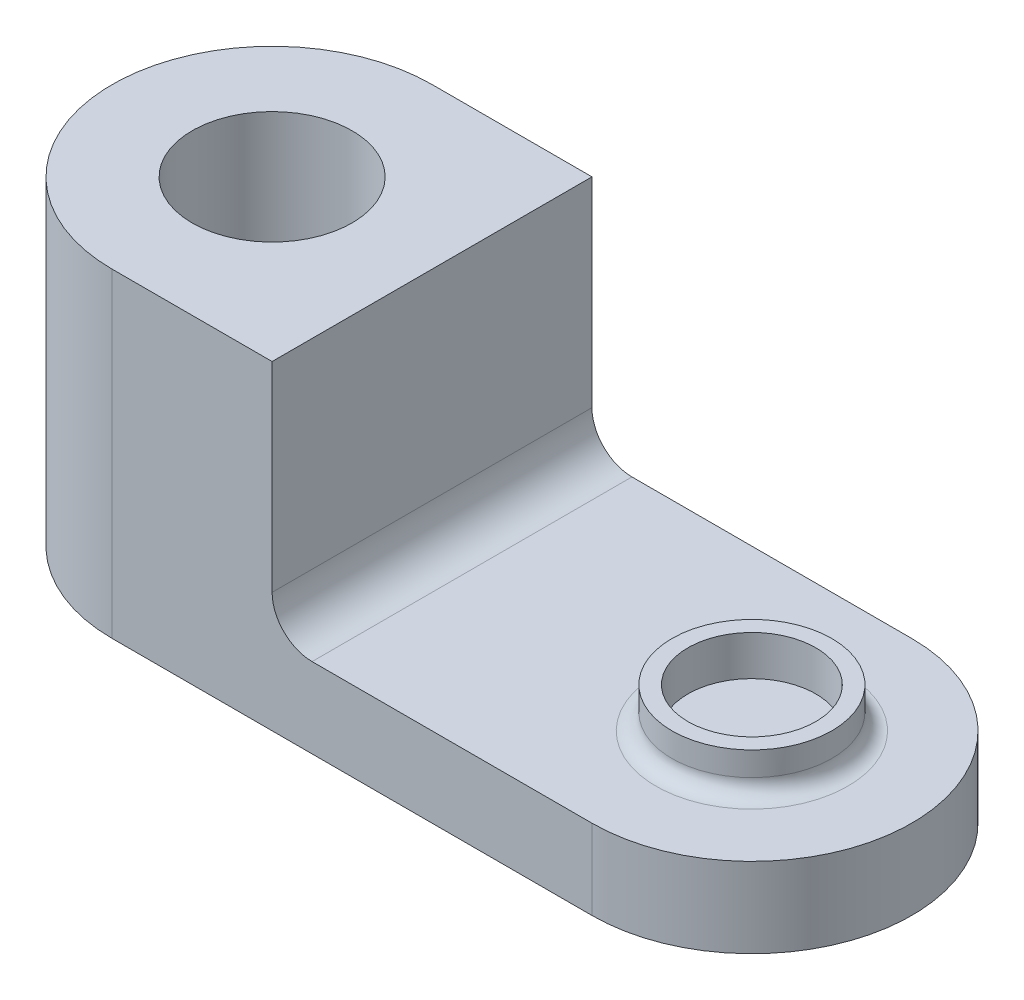
ISO-10303-21;
HEADER;
FILE_DESCRIPTION(('STEP AP214'),'2;1');
FILE_NAME('part.step','',(''),(''),'','','');
FILE_SCHEMA(('AUTOMOTIVE_DESIGN { 1 0 10303 214 1 1 1 1 }'));
ENDSEC;
DATA;
#1=APPLICATION_CONTEXT('core data for automotive mechanical design processes');
#2=APPLICATION_PROTOCOL_DEFINITION('international standard','automotive_design',2000,#1);
#3=PRODUCT_CONTEXT('',#1,'mechanical');
#4=PRODUCT('Part','Part','',(#3));
#5=PRODUCT_RELATED_PRODUCT_CATEGORY('part','',(#4));
#6=PRODUCT_DEFINITION_FORMATION('','',#4);
#7=PRODUCT_DEFINITION_CONTEXT('part definition',#1,'design');
#8=PRODUCT_DEFINITION('design','',#6,#7);
#9=PRODUCT_DEFINITION_SHAPE('','',#8);
#10=(LENGTH_UNIT() NAMED_UNIT(*) SI_UNIT(.MILLI.,.METRE.));
#11=(NAMED_UNIT(*) PLANE_ANGLE_UNIT() SI_UNIT($,.RADIAN.));
#12=(NAMED_UNIT(*) SI_UNIT($,.STERADIAN.) SOLID_ANGLE_UNIT());
#13=UNCERTAINTY_MEASURE_WITH_UNIT(LENGTH_MEASURE(1.E-05),#10,'distance_accuracy_value','');
#14=(GEOMETRIC_REPRESENTATION_CONTEXT(3) GLOBAL_UNCERTAINTY_ASSIGNED_CONTEXT((#13)) GLOBAL_UNIT_ASSIGNED_CONTEXT((#10,
#11,#12)) REPRESENTATION_CONTEXT('',''));
#15=CARTESIAN_POINT('',(0.,0.,0.));
#16=DIRECTION('',(0.,0.,1.));
#17=DIRECTION('',(1.,0.,0.));
#18=AXIS2_PLACEMENT_3D('',#15,#16,#17);
#19=CARTESIAN_POINT('',(80.,10.,20.));
#20=DIRECTION('',(0.,1.,0.));
#21=DIRECTION('',(0.,0.,1.));
#22=AXIS2_PLACEMENT_3D('',#19,#20,#21);
#23=CYLINDRICAL_SURFACE('',#22,20.);
#24=DIRECTION('',(0.,-1.,0.));
#25=VECTOR('',#24,1.);
#26=CARTESIAN_POINT('',(80.,10.,0.));
#27=LINE('',#26,#25);
#28=CARTESIAN_POINT('',(80.,10.,0.));
#29=VERTEX_POINT('',#28);
#30=CARTESIAN_POINT('',(80.,0.,0.));
#31=VERTEX_POINT('',#30);
#32=EDGE_CURVE('E146',#29,#31,#27,.T.);
#33=ORIENTED_EDGE('',*,*,#32,.F.);
#34=CARTESIAN_POINT('',(80.,10.,20.));
#35=DIRECTION('',(0.,-1.,0.));
#36=DIRECTION('',(0.,0.,-1.));
#37=AXIS2_PLACEMENT_3D('',#34,#35,#36);
#38=CIRCLE('',#37,20.);
#39=CARTESIAN_POINT('',(80.,10.,40.));
#40=VERTEX_POINT('',#39);
#41=EDGE_CURVE('E152',#40,#29,#38,.F.);
#42=ORIENTED_EDGE('',*,*,#41,.F.);
#43=DIRECTION('',(0.,1.,0.));
#44=VECTOR('',#43,1.);
#45=CARTESIAN_POINT('',(80.,0.,40.));
#46=LINE('',#45,#44);
#47=CARTESIAN_POINT('',(80.,0.,40.));
#48=VERTEX_POINT('',#47);
#49=EDGE_CURVE('E151',#48,#40,#46,.T.);
#50=ORIENTED_EDGE('',*,*,#49,.F.);
#51=CARTESIAN_POINT('',(80.,0.,20.));
#52=DIRECTION('',(0.,1.,0.));
#53=DIRECTION('',(0.,0.,1.));
#54=AXIS2_PLACEMENT_3D('',#51,#52,#53);
#55=CIRCLE('',#54,20.);
#56=EDGE_CURVE('E156',#31,#48,#55,.F.);
#57=ORIENTED_EDGE('',*,*,#56,.F.);
#58=EDGE_LOOP('',(#33,#42,#50,#57));
#59=FACE_BOUND('',#58,.T.);
#60=ADVANCED_FACE('F41',(#59),#23,.T.);
#61=CARTESIAN_POINT('',(20.,0.,20.));
#62=DIRECTION('',(0.,-1.,0.));
#63=DIRECTION('',(0.,0.,-1.));
#64=AXIS2_PLACEMENT_3D('',#61,#62,#63);
#65=CYLINDRICAL_SURFACE('',#64,20.);
#66=DIRECTION('',(0.,1.,0.));
#67=VECTOR('',#66,1.);
#68=CARTESIAN_POINT('',(20.,0.,0.));
#69=LINE('',#68,#67);
#70=CARTESIAN_POINT('',(20.,0.,0.));
#71=VERTEX_POINT('',#70);
#72=CARTESIAN_POINT('',(20.,40.,0.));
#73=VERTEX_POINT('',#72);
#74=EDGE_CURVE('E124',#71,#73,#69,.T.);
#75=ORIENTED_EDGE('',*,*,#74,.F.);
#76=CARTESIAN_POINT('',(20.,0.,20.));
#77=DIRECTION('',(0.,1.,0.));
#78=DIRECTION('',(0.,0.,1.));
#79=AXIS2_PLACEMENT_3D('',#76,#77,#78);
#80=CIRCLE('',#79,20.);
#81=CARTESIAN_POINT('',(20.,0.,40.));
#82=VERTEX_POINT('',#81);
#83=EDGE_CURVE('E144',#82,#71,#80,.F.);
#84=ORIENTED_EDGE('',*,*,#83,.F.);
#85=DIRECTION('',(0.,-1.,0.));
#86=VECTOR('',#85,1.);
#87=CARTESIAN_POINT('',(20.,0.,40.));
#88=LINE('',#87,#86);
#89=CARTESIAN_POINT('',(20.,40.,40.));
#90=VERTEX_POINT('',#89);
#91=EDGE_CURVE('E141',#90,#82,#88,.T.);
#92=ORIENTED_EDGE('',*,*,#91,.F.);
#93=CARTESIAN_POINT('',(20.,40.,20.));
#94=DIRECTION('',(0.,-1.,0.));
#95=DIRECTION('',(0.,0.,-1.));
#96=AXIS2_PLACEMENT_3D('',#93,#94,#95);
#97=CIRCLE('',#96,20.);
#98=EDGE_CURVE('E127',#73,#90,#97,.F.);
#99=ORIENTED_EDGE('',*,*,#98,.F.);
#100=EDGE_LOOP('',(#75,#84,#92,#99));
#101=FACE_BOUND('',#100,.T.);
#102=ADVANCED_FACE('F176',(#101),#65,.T.);
#103=CARTESIAN_POINT('',(0.,0.,40.));
#104=DIRECTION('',(0.,1.,0.));
#105=DIRECTION('',(0.,0.,1.));
#106=AXIS2_PLACEMENT_3D('',#103,#104,#105);
#107=PLANE('',#106);
#108=CARTESIAN_POINT('',(20.,0.,20.));
#109=DIRECTION('',(0.,1.,0.));
#110=DIRECTION('',(0.,0.,1.));
#111=AXIS2_PLACEMENT_3D('',#108,#109,#110);
#112=CIRCLE('',#111,10.);
#113=CARTESIAN_POINT('',(20.,0.,30.));
#114=VERTEX_POINT('',#113);
#115=EDGE_CURVE('E133',#114,#114,#112,.T.);
#116=ORIENTED_EDGE('',*,*,#115,.T.);
#117=EDGE_LOOP('',(#116));
#118=FACE_BOUND('',#117,.T.);
#119=DIRECTION('',(1.,0.,0.));
#120=VECTOR('',#119,1.);
#121=CARTESIAN_POINT('',(0.,0.,0.));
#122=LINE('',#121,#120);
#123=EDGE_CURVE('E132',#71,#31,#122,.T.);
#124=ORIENTED_EDGE('',*,*,#123,.T.);
#125=ORIENTED_EDGE('',*,*,#56,.T.);
#126=DIRECTION('',(1.,0.,0.));
#127=VECTOR('',#126,1.);
#128=CARTESIAN_POINT('',(0.,0.,40.));
#129=LINE('',#128,#127);
#130=EDGE_CURVE('E136',#82,#48,#129,.T.);
#131=ORIENTED_EDGE('',*,*,#130,.F.);
#132=ORIENTED_EDGE('',*,*,#83,.T.);
#133=EDGE_LOOP('',(#124,#125,#131,#132));
#134=FACE_BOUND('',#133,.T.);
#135=ADVANCED_FACE('F189',(#118,#134),#107,.F.);
#136=CARTESIAN_POINT('',(40.,10.,40.));
#137=DIRECTION('',(0.,-1.,0.));
#138=DIRECTION('',(0.,0.,-1.));
#139=AXIS2_PLACEMENT_3D('',#136,#137,#138);
#140=PLANE('',#139);
#141=CARTESIAN_POINT('',(80.,10.,20.));
#142=DIRECTION('',(0.,-1.,0.));
#143=DIRECTION('',(0.,0.,-1.));
#144=AXIS2_PLACEMENT_3D('',#141,#142,#143);
#145=CIRCLE('',#144,12.);
#146=CARTESIAN_POINT('',(80.,10.,8.00000000000001));
#147=VERTEX_POINT('',#146);
#148=EDGE_CURVE('E11',#147,#147,#145,.T.);
#149=ORIENTED_EDGE('',*,*,#148,.T.);
#150=EDGE_LOOP('',(#149));
#151=FACE_BOUND('',#150,.T.);
#152=DIRECTION('',(-1.,0.,0.));
#153=VECTOR('',#152,1.);
#154=CARTESIAN_POINT('',(40.,10.,0.));
#155=LINE('',#154,#153);
#156=CARTESIAN_POINT('',(45.,10.,0.));
#157=VERTEX_POINT('',#156);
#158=EDGE_CURVE('E131',#29,#157,#155,.T.);
#159=ORIENTED_EDGE('',*,*,#158,.T.);
#160=DIRECTION('',(0.,0.,-1.));
#161=VECTOR('',#160,1.);
#162=CARTESIAN_POINT('',(45.,10.,40.));
#163=LINE('',#162,#161);
#164=CARTESIAN_POINT('',(45.,10.,40.));
#165=VERTEX_POINT('',#164);
#166=EDGE_CURVE('E65',#157,#165,#163,.F.);
#167=ORIENTED_EDGE('',*,*,#166,.T.);
#168=DIRECTION('',(-1.,0.,0.));
#169=VECTOR('',#168,1.);
#170=CARTESIAN_POINT('',(40.,10.,40.));
#171=LINE('',#170,#169);
#172=EDGE_CURVE('E111',#40,#165,#171,.T.);
#173=ORIENTED_EDGE('',*,*,#172,.F.);
#174=ORIENTED_EDGE('',*,*,#41,.T.);
#175=EDGE_LOOP('',(#159,#167,#173,#174));
#176=FACE_BOUND('',#175,.T.);
#177=ADVANCED_FACE('F200',(#151,#176),#140,.F.);
#178=CARTESIAN_POINT('',(40.,40.,40.));
#179=DIRECTION('',(-1.,0.,0.));
#180=DIRECTION('',(0.,0.,1.));
#181=AXIS2_PLACEMENT_3D('',#178,#179,#180);
#182=PLANE('',#181);
#183=DIRECTION('',(0.,1.,0.));
#184=VECTOR('',#183,1.);
#185=CARTESIAN_POINT('',(40.,40.,40.));
#186=LINE('',#185,#184);
#187=CARTESIAN_POINT('',(40.,15.,40.));
#188=VERTEX_POINT('',#187);
#189=CARTESIAN_POINT('',(40.,40.,40.));
#190=VERTEX_POINT('',#189);
#191=EDGE_CURVE('E105',#188,#190,#186,.T.);
#192=ORIENTED_EDGE('',*,*,#191,.F.);
#193=DIRECTION('',(0.,0.,-1.));
#194=VECTOR('',#193,1.);
#195=CARTESIAN_POINT('',(40.,15.,0.));
#196=LINE('',#195,#194);
#197=CARTESIAN_POINT('',(40.,15.,0.));
#198=VERTEX_POINT('',#197);
#199=EDGE_CURVE('E158',#188,#198,#196,.T.);
#200=ORIENTED_EDGE('',*,*,#199,.T.);
#201=DIRECTION('',(0.,1.,0.));
#202=VECTOR('',#201,1.);
#203=CARTESIAN_POINT('',(40.,40.,0.));
#204=LINE('',#203,#202);
#205=CARTESIAN_POINT('',(40.,40.,0.));
#206=VERTEX_POINT('',#205);
#207=EDGE_CURVE('E116',#198,#206,#204,.T.);
#208=ORIENTED_EDGE('',*,*,#207,.T.);
#209=DIRECTION('',(0.,0.,-1.));
#210=VECTOR('',#209,1.);
#211=CARTESIAN_POINT('',(40.,40.,40.));
#212=LINE('',#211,#210);
#213=EDGE_CURVE('E119',#190,#206,#212,.T.);
#214=ORIENTED_EDGE('',*,*,#213,.F.);
#215=EDGE_LOOP('',(#192,#200,#208,#214));
#216=FACE_BOUND('',#215,.T.);
#217=ADVANCED_FACE('F120',(#216),#182,.F.);
#218=CARTESIAN_POINT('',(0.,40.,40.));
#219=DIRECTION('',(0.,-1.,0.));
#220=DIRECTION('',(0.,0.,-1.));
#221=AXIS2_PLACEMENT_3D('',#218,#219,#220);
#222=PLANE('',#221);
#223=CARTESIAN_POINT('',(20.,40.,20.));
#224=DIRECTION('',(0.,1.,0.));
#225=DIRECTION('',(0.,0.,1.));
#226=AXIS2_PLACEMENT_3D('',#223,#224,#225);
#227=CIRCLE('',#226,10.);
#228=CARTESIAN_POINT('',(20.,40.,30.));
#229=VERTEX_POINT('',#228);
#230=EDGE_CURVE('E244',#229,#229,#227,.T.);
#231=ORIENTED_EDGE('',*,*,#230,.F.);
#232=EDGE_LOOP('',(#231));
#233=FACE_BOUND('',#232,.T.);
#234=DIRECTION('',(-1.,0.,0.));
#235=VECTOR('',#234,1.);
#236=CARTESIAN_POINT('',(0.,40.,0.));
#237=LINE('',#236,#235);
#238=EDGE_CURVE('E139',#206,#73,#237,.T.);
#239=ORIENTED_EDGE('',*,*,#238,.T.);
#240=ORIENTED_EDGE('',*,*,#98,.T.);
#241=DIRECTION('',(-1.,0.,0.));
#242=VECTOR('',#241,1.);
#243=CARTESIAN_POINT('',(0.,40.,40.));
#244=LINE('',#243,#242);
#245=EDGE_CURVE('E107',#190,#90,#244,.T.);
#246=ORIENTED_EDGE('',*,*,#245,.F.);
#247=ORIENTED_EDGE('',*,*,#213,.T.);
#248=EDGE_LOOP('',(#239,#240,#246,#247));
#249=FACE_BOUND('',#248,.T.);
#250=ADVANCED_FACE('F123',(#233,#249),#222,.F.);
#251=CARTESIAN_POINT('',(0.,0.,40.));
#252=DIRECTION('',(0.,0.,-1.));
#253=DIRECTION('',(-1.,0.,0.));
#254=AXIS2_PLACEMENT_3D('',#251,#252,#253);
#255=PLANE('',#254);
#256=ORIENTED_EDGE('',*,*,#130,.T.);
#257=ORIENTED_EDGE('',*,*,#49,.T.);
#258=ORIENTED_EDGE('',*,*,#172,.T.);
#259=CARTESIAN_POINT('',(45.,15.,40.));
#260=DIRECTION('',(0.,0.,-1.));
#261=DIRECTION('',(-1.,0.,0.));
#262=AXIS2_PLACEMENT_3D('',#259,#260,#261);
#263=CIRCLE('',#262,5.);
#264=EDGE_CURVE('E109',#165,#188,#263,.T.);
#265=ORIENTED_EDGE('',*,*,#264,.T.);
#266=ORIENTED_EDGE('',*,*,#191,.T.);
#267=ORIENTED_EDGE('',*,*,#245,.T.);
#268=ORIENTED_EDGE('',*,*,#91,.T.);
#269=EDGE_LOOP('',(#256,#257,#258,#265,#266,#267,#268));
#270=FACE_BOUND('',#269,.T.);
#271=ADVANCED_FACE('F104',(#270),#255,.F.);
#272=CARTESIAN_POINT('',(0.,0.,0.));
#273=DIRECTION('',(0.,0.,-1.));
#274=DIRECTION('',(-1.,0.,0.));
#275=AXIS2_PLACEMENT_3D('',#272,#273,#274);
#276=PLANE('',#275);
#277=ORIENTED_EDGE('',*,*,#158,.F.);
#278=ORIENTED_EDGE('',*,*,#32,.T.);
#279=ORIENTED_EDGE('',*,*,#123,.F.);
#280=ORIENTED_EDGE('',*,*,#74,.T.);
#281=ORIENTED_EDGE('',*,*,#238,.F.);
#282=ORIENTED_EDGE('',*,*,#207,.F.);
#283=CARTESIAN_POINT('',(45.,15.,0.));
#284=DIRECTION('',(0.,0.,-1.));
#285=DIRECTION('',(-1.,0.,0.));
#286=AXIS2_PLACEMENT_3D('',#283,#284,#285);
#287=CIRCLE('',#286,5.);
#288=EDGE_CURVE('E57',#198,#157,#287,.F.);
#289=ORIENTED_EDGE('',*,*,#288,.T.);
#290=EDGE_LOOP('',(#277,#278,#279,#280,#281,#282,#289));
#291=FACE_BOUND('',#290,.T.);
#292=ADVANCED_FACE('F207',(#291),#276,.T.);
#293=CARTESIAN_POINT('',(20.,0.,20.));
#294=DIRECTION('',(0.,1.,0.));
#295=DIRECTION('',(0.,0.,1.));
#296=AXIS2_PLACEMENT_3D('',#293,#294,#295);
#297=CYLINDRICAL_SURFACE('',#296,10.);
#298=ORIENTED_EDGE('',*,*,#115,.F.);
#299=EDGE_LOOP('',(#298));
#300=FACE_BOUND('',#299,.T.);
#301=ORIENTED_EDGE('',*,*,#230,.T.);
#302=EDGE_LOOP('',(#301));
#303=FACE_BOUND('',#302,.T.);
#304=ADVANCED_FACE('F215',(#300,#303),#297,.F.);
#305=CARTESIAN_POINT('',(80.,15.,20.));
#306=DIRECTION('',(0.,1.,0.));
#307=DIRECTION('',(0.,0.,1.));
#308=AXIS2_PLACEMENT_3D('',#305,#306,#307);
#309=PLANE('',#308);
#310=CARTESIAN_POINT('',(80.,15.,20.));
#311=DIRECTION('',(0.,1.,0.));
#312=DIRECTION('',(0.,0.,1.));
#313=AXIS2_PLACEMENT_3D('',#310,#311,#312);
#314=CIRCLE('',#313,9.99999999999999);
#315=CARTESIAN_POINT('',(80.,15.,30.));
#316=VERTEX_POINT('',#315);
#317=EDGE_CURVE('E240',#316,#316,#314,.T.);
#318=ORIENTED_EDGE('',*,*,#317,.T.);
#319=EDGE_LOOP('',(#318));
#320=FACE_BOUND('',#319,.T.);
#321=CARTESIAN_POINT('',(80.,15.,20.));
#322=DIRECTION('',(0.,1.,0.));
#323=DIRECTION('',(0.,0.,1.));
#324=AXIS2_PLACEMENT_3D('',#321,#322,#323);
#325=CIRCLE('',#324,8.00000000000001);
#326=CARTESIAN_POINT('',(80.,15.,28.));
#327=VERTEX_POINT('',#326);
#328=EDGE_CURVE('E235',#327,#327,#325,.T.);
#329=ORIENTED_EDGE('',*,*,#328,.F.);
#330=EDGE_LOOP('',(#329));
#331=FACE_BOUND('',#330,.T.);
#332=ADVANCED_FACE('F216',(#320,#331),#309,.T.);
#333=CARTESIAN_POINT('',(80.,15.,20.));
#334=DIRECTION('',(0.,-1.,0.));
#335=DIRECTION('',(0.,0.,-1.));
#336=AXIS2_PLACEMENT_3D('',#333,#334,#335);
#337=CYLINDRICAL_SURFACE('',#336,9.99999999999999);
#338=CARTESIAN_POINT('',(80.,12.,20.));
#339=DIRECTION('',(0.,-1.,0.));
#340=DIRECTION('',(0.,0.,-1.));
#341=AXIS2_PLACEMENT_3D('',#338,#339,#340);
#342=CIRCLE('',#341,9.99999999999999);
#343=CARTESIAN_POINT('',(80.,12.,10.));
#344=VERTEX_POINT('',#343);
#345=EDGE_CURVE('E47',#344,#344,#342,.F.);
#346=ORIENTED_EDGE('',*,*,#345,.T.);
#347=EDGE_LOOP('',(#346));
#348=FACE_BOUND('',#347,.T.);
#349=ORIENTED_EDGE('',*,*,#317,.F.);
#350=EDGE_LOOP('',(#349));
#351=FACE_BOUND('',#350,.T.);
#352=ADVANCED_FACE('F164',(#348,#351),#337,.T.);
#353=CARTESIAN_POINT('',(80.,15.,20.));
#354=DIRECTION('',(0.,-1.,0.));
#355=DIRECTION('',(0.,0.,-1.));
#356=AXIS2_PLACEMENT_3D('',#353,#354,#355);
#357=CYLINDRICAL_SURFACE('',#356,8.00000000000001);
#358=ORIENTED_EDGE('',*,*,#328,.T.);
#359=EDGE_LOOP('',(#358));
#360=FACE_BOUND('',#359,.T.);
#361=CARTESIAN_POINT('',(80.,10.,20.));
#362=DIRECTION('',(0.,1.,0.));
#363=DIRECTION('',(0.,0.,1.));
#364=AXIS2_PLACEMENT_3D('',#361,#362,#363);
#365=CIRCLE('',#364,8.00000000000001);
#366=CARTESIAN_POINT('',(80.,10.,28.));
#367=VERTEX_POINT('',#366);
#368=EDGE_CURVE('E233',#367,#367,#365,.T.);
#369=ORIENTED_EDGE('',*,*,#368,.F.);
#370=EDGE_LOOP('',(#369));
#371=FACE_BOUND('',#370,.T.);
#372=ADVANCED_FACE('F218',(#360,#371),#357,.F.);
#373=ORIENTED_EDGE('',*,*,#368,.T.);
#374=EDGE_LOOP('',(#373));
#375=FACE_BOUND('',#374,.T.);
#376=ADVANCED_FACE('F173',(#375),#140,.F.);
#377=CARTESIAN_POINT('',(45.,15.,40.));
#378=DIRECTION('',(0.,0.,1.));
#379=DIRECTION('',(1.,0.,0.));
#380=AXIS2_PLACEMENT_3D('',#377,#378,#379);
#381=CYLINDRICAL_SURFACE('',#380,5.);
#382=ORIENTED_EDGE('',*,*,#264,.F.);
#383=ORIENTED_EDGE('',*,*,#166,.F.);
#384=ORIENTED_EDGE('',*,*,#288,.F.);
#385=ORIENTED_EDGE('',*,*,#199,.F.);
#386=EDGE_LOOP('',(#382,#383,#384,#385));
#387=FACE_BOUND('',#386,.T.);
#388=ADVANCED_FACE('F166',(#387),#381,.F.);
#389=CARTESIAN_POINT('',(80.,12.,20.));
#390=DIRECTION('',(0.,-1.,0.));
#391=DIRECTION('',(0.,0.,-1.));
#392=AXIS2_PLACEMENT_3D('',#389,#390,#391);
#393=TOROIDAL_SURFACE('',#392,12.,2.);
#394=ORIENTED_EDGE('',*,*,#148,.F.);
#395=EDGE_LOOP('',(#394));
#396=FACE_BOUND('',#395,.T.);
#397=ORIENTED_EDGE('',*,*,#345,.F.);
#398=EDGE_LOOP('',(#397));
#399=FACE_BOUND('',#398,.T.);
#400=ADVANCED_FACE('F43',(#396,#399),#393,.F.);
#401=CLOSED_SHELL('',(#60,#102,#135,#177,#217,#250,#271,#292,#304,#332,#352,#372,#376,#388,#400));
#402=MANIFOLD_SOLID_BREP('B2',#401);
#403=ADVANCED_BREP_SHAPE_REPRESENTATION('',(#18,#402),#14);
#404=SHAPE_DEFINITION_REPRESENTATION(#9,#403);
ENDSEC;
END-ISO-10303-21;
